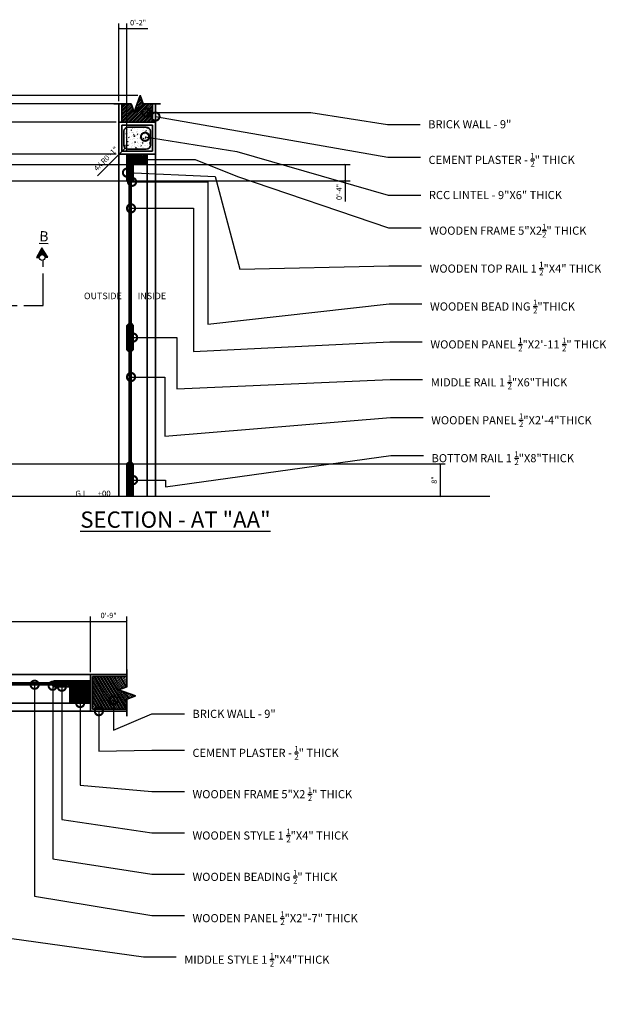
# Model space of a CAD drawing. Units: inches. Extents: x 1926 to 2169, y 1541 to 1783.
# Tile 3 of 3: x 2025 to 2169, y 1541 to 1783. Entities that reach past the tile are written whole.
import ezdxf
from ezdxf import colors
from ezdxf.entities.mleader import LeaderData, LeaderLine
from ezdxf.math import Vec2, Vec3

# ---------------------------------------------------------------- set-up
doc = ezdxf.new("R2010")
doc.units = ezdxf.units.IN
doc.linetypes.add('CENTER', pattern=[50.8, 31.75, -6.35, 6.35, -6.35])
for name, color, linetype, lineweight in [('A-ANNO-DIMS', 2, 'Continuous', 18), ('A-ANNO-SECT', 1, 'CENTER', 25), ('A-ANNO-SYMB', 1, 'Continuous', 25), ('A-ANNO-TEXT', 3, 'Continuous', 25), ('A-DETL', 7, 'Continuous', 35), ('A-DETL-PATT', 8, 'Continuous', 18)]:
    doc.layers.add(name, color=color, linetype=linetype, lineweight=lineweight)
doc.styles.get("Standard").update_dxf_attribs({"font": 'arial.ttf'})
doc.dimstyles.new('ISO-25', dxfattribs={"dimtxt": 1.3125, "dimasz": 0.375, "dimexe": 1.25, "dimexo": 0.625, "dimtad": 1, "dimzin": 3, "dimlunit": 4, "dimtxsty": 'Standard', "dimblk": 'ARCHTICK', "dimcen": 0.09, "dimadec": 0, "dimazin": 0, "dimtfac": 1, "dimtofl": 0, "dimtmove": 0, "dimatfit": 3, "dimfxl": 1, "dimarcsym": 0})

# ---------------------------------------------------------------- blocks, each defined once
blk = doc.blocks.new('_DotSmall')
at = {"color": 0, "linetype": 'ByBlock', "const_width": 0.5}
blk.add_lwpolyline([(-0.0625, 0, 1), (0.0625, 0, 1)], format="xyb", close=True, dxfattribs=at)
blk = doc.blocks.new('_ArchTick')
at = {"color": 0, "linetype": 'ByBlock', "const_width": 0.15}
blk.add_lwpolyline([(-0.5, -0.5), (0.5, 0.5)], dxfattribs=at)
blk = doc.blocks.new('*D24')
at = {"layer": 'A-ANNO-DIMS', "color": 0, "lineweight": -2, "transparency": 16777216}
for p, q in [((1974.41, 1673.81), (2129.74, 1673.81)), ((2128.49, 1673.81), (2128.49, 1665.81)), ((2134.77, 1665.81), (2127.24, 1665.81))]:
    blk.add_line(p, q, dxfattribs=at)
at = {"layer": 'DEFPOINTS', "color": 0, "transparency": 16777216}
for p in [(1973.78, 1673.81), (2128.49, 1665.81), (2135.4, 1665.81)]:
    blk.add_point(p, dxfattribs=at)
at = {"layer": 'A-ANNO-DIMS', "color": 0, "lineweight": -2, "transparency": 16777216, "xscale": 0.375, "yscale": 0.375, "zscale": 0.375}
for p, rotation in [((2128.49, 1673.81), 90), ((2128.49, 1665.81), 270)]:
    blk.add_blockref('_ArchTick', p, dxfattribs=dict(at, rotation=rotation))
at = {"layer": 'A-ANNO-DIMS', "color": 0, "transparency": 16777216, "insert": (2127.2, 1669.81), "char_height": 1.312, "attachment_point": 5, "rotation": 90}
blk.add_mtext('8"', dxfattribs=at)
blk = doc.blocks.new('*D28')
at = {"layer": 'A-ANNO-DIMS', "color": 0, "lineweight": -2, "transparency": 16777216}
for p, q in [((1966.66, 1749.81), (1954.13, 1749.81)), ((1955.38, 1749.81), (1955.38, 1665.81)), ((2140.71, 1665.81), (1954.13, 1665.81))]:
    blk.add_line(p, q, dxfattribs=at)
at = {"layer": 'DEFPOINTS', "color": 0, "transparency": 16777216}
for p in [(1967.28, 1749.81), (1955.38, 1665.81), (2141.33, 1665.81)]:
    blk.add_point(p, dxfattribs=at)
at = {"layer": 'A-ANNO-DIMS', "color": 0, "lineweight": -2, "transparency": 16777216, "xscale": 0.375, "yscale": 0.375, "zscale": 0.375}
for p, rotation in [((1955.38, 1749.81), 90), ((1955.38, 1665.81), 270)]:
    blk.add_blockref('_ArchTick', p, dxfattribs=dict(at, rotation=rotation))
at = {"layer": 'A-ANNO-DIMS', "color": 0, "transparency": 16777216, "insert": (1954.09, 1707.81), "char_height": 1.312, "attachment_point": 5, "rotation": 90}
blk.add_mtext('7\'-0"', dxfattribs=at)
blk = doc.blocks.new('*D32')
at = {"layer": 'A-ANNO-DIMS', "color": 0, "lineweight": -2, "transparency": 16777216}
for p, q in [((2013.41, 1747.31), (2106.38, 1747.31)), ((2105.13, 1747.31), (2105.13, 1743.31)), ((2009.41, 1743.31), (2106.38, 1743.31)), ((2105.13, 1743.31), (2105.13, 1738.19))]:
    blk.add_line(p, q, dxfattribs=at)
at = {"layer": 'DEFPOINTS', "color": 0, "transparency": 16777216}
for p in [(2012.78, 1747.31), (2008.78, 1743.31), (2105.13, 1743.31)]:
    blk.add_point(p, dxfattribs=at)
at = {"layer": 'A-ANNO-DIMS', "color": 0, "lineweight": -2, "transparency": 16777216, "xscale": 0.375, "yscale": 0.375, "zscale": 0.375}
for p, rotation in [((2105.13, 1747.31), 90), ((2105.13, 1743.31), 270)]:
    blk.add_blockref('_ArchTick', p, dxfattribs=dict(at, rotation=rotation))
at = {"layer": 'A-ANNO-DIMS', "color": 0, "transparency": 16777216, "insert": (2103.84, 1740.56), "char_height": 1.312, "attachment_point": 5, "rotation": 90}
blk.add_mtext('0\'-4"', dxfattribs=at)
blk = doc.blocks.new('*D35')
at = {"layer": 'A-ANNO-DIMS', "color": 0, "lineweight": -2, "transparency": 16777216}
for p, q in [((2054.17, 1764.25), (1935.51, 1764.25)), ((1936.76, 1665.81), (1936.76, 1764.25)), ((2048.92, 1665.81), (1935.51, 1665.81))]:
    blk.add_line(p, q, dxfattribs=at)
at = {"layer": 'DEFPOINTS', "color": 0, "transparency": 16777216}
for p in [(1936.76, 1764.25), (2054.79, 1764.25), (2049.54, 1665.81)]:
    blk.add_point(p, dxfattribs=at)
at = {"layer": 'A-ANNO-DIMS', "color": 0, "lineweight": -2, "transparency": 16777216, "xscale": 0.375, "yscale": 0.375, "zscale": 0.375}
for p, rotation in [((1936.76, 1764.25), 90), ((1936.76, 1665.81), 270)]:
    blk.add_blockref('_ArchTick', p, dxfattribs=dict(at, rotation=rotation))
at = {"layer": 'A-ANNO-DIMS', "color": 0, "transparency": 16777216, "insert": (1935.45, 1715.03), "char_height": 1.312, "attachment_point": 5, "rotation": 90}
blk.add_mtext('8\'-2 1/2"', dxfattribs=at)
blk = doc.blocks.new('*D36')
at = {"layer": 'A-ANNO-DIMS', "color": 0, "lineweight": -2, "transparency": 16777216}
for p, q in [((2049.54, 1762.82), (2049.54, 1781.93)), ((2049.54, 1780.68), (2051.54, 1780.68)), ((2051.54, 1750.43), (2051.54, 1781.93)), ((2051.54, 1780.68), (2056.65, 1780.68))]:
    blk.add_line(p, q, dxfattribs=at)
at = {"layer": 'DEFPOINTS', "color": 0, "transparency": 16777216}
for p in [(2051.54, 1780.68), (2049.54, 1762.19), (2051.54, 1749.81)]:
    blk.add_point(p, dxfattribs=at)
at = {"layer": 'A-ANNO-DIMS', "color": 0, "lineweight": -2, "transparency": 16777216, "xscale": 0.375, "yscale": 0.375, "zscale": 0.375, "rotation": 180}
blk.add_blockref('_ArchTick', (2049.54, 1780.68), dxfattribs=at)
at = {"layer": 'A-ANNO-DIMS', "color": 0, "lineweight": -2, "transparency": 16777216, "xscale": 0.375, "yscale": 0.375, "zscale": 0.375}
blk.add_blockref('_ArchTick', (2051.54, 1780.68), dxfattribs=at)
at = {"layer": 'A-ANNO-DIMS', "color": 0, "transparency": 16777216, "insert": (2054.28, 1781.97), "char_height": 1.312, "attachment_point": 5}
blk.add_mtext('0\'-2"', dxfattribs=at)
blk = doc.blocks.new('*D37')
at = {"layer": 'A-ANNO-DIMS', "color": 0, "lineweight": -2, "transparency": 16777216}
for p, q in [((2048.92, 1757.73), (1935.51, 1757.73)), ((1936.76, 1749.81), (1936.76, 1757.73)), ((2048.92, 1749.81), (1935.51, 1749.81))]:
    blk.add_line(p, q, dxfattribs=at)
at = {"layer": 'DEFPOINTS', "color": 0, "transparency": 16777216}
for p in [(1936.76, 1757.73), (2049.54, 1757.73), (2049.54, 1749.81)]:
    blk.add_point(p, dxfattribs=at)
at = {"layer": 'A-ANNO-DIMS', "color": 0, "lineweight": -2, "transparency": 16777216, "xscale": 0.375, "yscale": 0.375, "zscale": 0.375}
for p, rotation in [((1936.76, 1757.73), 90), ((1936.76, 1749.81), 270)]:
    blk.add_blockref('_ArchTick', p, dxfattribs=dict(at, rotation=rotation))
at = {"layer": 'A-ANNO-DIMS', "color": 0, "transparency": 16777216, "insert": (1935.46, 1753.77), "char_height": 1.312, "attachment_point": 5, "rotation": 90}
blk.add_mtext('0\'-8"', dxfattribs=at)
blk = doc.blocks.new('*D38')
at = {"layer": 'A-ANNO-DIMS', "color": 0, "lineweight": -2, "transparency": 16777216}
for p, q in [((1936.76, 1762.19), (1936.76, 1770.36)), ((2048.92, 1762.19), (1935.51, 1762.19)), ((1936.76, 1757.73), (1936.76, 1762.19)), ((2048.92, 1757.73), (1935.51, 1757.73))]:
    blk.add_line(p, q, dxfattribs=at)
at = {"layer": 'DEFPOINTS', "color": 0, "transparency": 16777216}
for p in [(1936.76, 1762.19), (2049.54, 1762.19), (2049.54, 1757.73)]:
    blk.add_point(p, dxfattribs=at)
at = {"layer": 'A-ANNO-DIMS', "color": 0, "lineweight": -2, "transparency": 16777216, "xscale": 0.375, "yscale": 0.375, "zscale": 0.375}
for p, rotation in [((1936.76, 1762.19), 90), ((1936.76, 1757.73), 270)]:
    blk.add_blockref('_ArchTick', p, dxfattribs=dict(at, rotation=rotation))
at = {"layer": 'A-ANNO-DIMS', "color": 0, "transparency": 16777216, "insert": (1935.45, 1766.46), "char_height": 1.312, "attachment_point": 5, "rotation": 90}
blk.add_mtext('0\'-4 1/2"', dxfattribs=at)
blk = doc.blocks.new('*D40')
at = {"layer": 'A-ANNO-DIMS', "color": 0, "lineweight": -2, "transparency": 16777216}
for p, q in [((1952.54, 1622.67), (1952.54, 1636.34)), ((1952.54, 1635.09), (2042.54, 1635.09)), ((2042.54, 1622.67), (2042.54, 1636.34))]:
    blk.add_line(p, q, dxfattribs=at)
at = {"layer": 'DEFPOINTS', "color": 0, "transparency": 16777216}
for p in [(2042.54, 1635.09), (1952.54, 1622.04), (2042.54, 1622.04)]:
    blk.add_point(p, dxfattribs=at)
at = {"layer": 'A-ANNO-DIMS', "color": 0, "lineweight": -2, "transparency": 16777216, "xscale": 0.375, "yscale": 0.375, "zscale": 0.375, "rotation": 180}
blk.add_blockref('_ArchTick', (1952.54, 1635.09), dxfattribs=at)
at = {"layer": 'A-ANNO-DIMS', "color": 0, "lineweight": -2, "transparency": 16777216, "xscale": 0.375, "yscale": 0.375, "zscale": 0.375}
blk.add_blockref('_ArchTick', (2042.54, 1635.09), dxfattribs=at)
at = {"layer": 'A-ANNO-DIMS', "color": 0, "transparency": 16777216, "insert": (1997.54, 1636.39), "char_height": 1.312, "attachment_point": 5}
blk.add_mtext('7\'-6"', dxfattribs=at)
blk = doc.blocks.new('*D41')
at = {"layer": 'A-ANNO-DIMS', "color": 0, "lineweight": -2, "transparency": 16777216}
for p, q in [((2042.54, 1622.67), (2042.54, 1636.34)), ((2042.54, 1635.09), (2051.54, 1635.09)), ((2051.54, 1622.67), (2051.54, 1636.34))]:
    blk.add_line(p, q, dxfattribs=at)
at = {"layer": 'DEFPOINTS', "color": 0, "transparency": 16777216}
for p in [(2051.54, 1635.09), (2042.54, 1622.04), (2051.54, 1622.04)]:
    blk.add_point(p, dxfattribs=at)
at = {"layer": 'A-ANNO-DIMS', "color": 0, "lineweight": -2, "transparency": 16777216, "xscale": 0.375, "yscale": 0.375, "zscale": 0.375, "rotation": 180}
blk.add_blockref('_ArchTick', (2042.54, 1635.09), dxfattribs=at)
at = {"layer": 'A-ANNO-DIMS', "color": 0, "lineweight": -2, "transparency": 16777216, "xscale": 0.375, "yscale": 0.375, "zscale": 0.375}
blk.add_blockref('_ArchTick', (2051.54, 1635.09), dxfattribs=at)
at = {"layer": 'A-ANNO-DIMS', "color": 0, "transparency": 16777216, "insert": (2047.04, 1636.39), "char_height": 1.312, "attachment_point": 5}
blk.add_mtext('0\'-9"', dxfattribs=at)
blk = doc.blocks.new('*D44')
at = {"layer": 'A-ANNO-DIMS', "color": 0, "lineweight": -2, "transparency": 16777216}
for p, q in [((2044.28, 1744.55), (2051.08, 1751.35)), ((2051.7, 1752.06), (2051.88, 1752.06)), ((2051.79, 1751.97), (2051.79, 1752.15))]:
    blk.add_line(p, q, dxfattribs=at)
at = {"layer": 'DEFPOINTS', "color": 0, "transparency": 16777216}
for p in [(2051.08, 1751.35), (2051.79, 1752.06)]:
    blk.add_point(p, dxfattribs=at)
at = {"layer": 'A-ANNO-DIMS', "color": 0, "lineweight": -2, "transparency": 16777216, "xscale": 0.375, "yscale": 0.375, "zscale": 0.375, "rotation": 45.01442306261743}
blk.add_blockref('_ArchTick', (2051.08, 1751.35), dxfattribs=at)
at = {"layer": 'A-ANNO-DIMS', "color": 0, "transparency": 16777216, "insert": (2046.5, 1748.6), "char_height": 1.312, "attachment_point": 5, "rotation": 45.0144}
blk.add_mtext('4X R0\'-1"', dxfattribs=at)

msp = doc.modelspace()

# ---------------------------------------------------------------- hatches: boundary and pattern name
at = {"layer": 'A-ANNO-SYMB'}
h = msp.add_hatch(color=256, dxfattribs=at)
h.dxf.hatch_style = 1
h.paths.add_polyline_path([(2031.409, 1724.514), (2032.103, 1724.566), (2030.609, 1726.871), (2029.289, 1724.461), (2029.985, 1724.461, -0.9636592)])
h = msp.add_hatch(dxfattribs=at)
h.set_pattern_fill('ANGLE', color=256, angle=90)
h.set_pattern_definition([(90, (3705.052, -295.39), (-6.985, 4e-16), [5.08, -1.905]), (180, (3705.052, -295.39), (-9e-16, -6.985), [5.08, -1.905])])
h.paths.add_polyline_path([(2054.821, 1719.063), (2053.501, 1716.653), (2054.197, 1716.653, -0.4142136), (2054.91, 1717.366, -0.3926966), (2055.621, 1716.706), (2056.315, 1716.757)])
at = {"layer": 'A-DETL-PATT'}
h = msp.add_hatch(dxfattribs=at)
h.set_pattern_fill('ANSI31', color=256, scale=0.1)
h.paths.add_polyline_path([(2053.29, 1760.129), (2052.54, 1762.19), (2050.29, 1762.19), (2050.29, 1757.726), (2057.79, 1757.726), (2057.79, 1762.19), (2055.54, 1762.19), (2054.79, 1764.251)])
h = msp.add_hatch(dxfattribs=at)
h.set_pattern_fill('AR-SAND', color=256)
h.paths.add_polyline_path([(2057.29, 1755.476, 0.4142136), (2056.29, 1756.476), (2051.79, 1756.476, 0.4142136), (2050.79, 1755.476), (2050.79, 1752.056, 0.4142136), (2051.79, 1751.056), (2056.29, 1751.056, 0.4142136), (2057.29, 1752.056)])
h = msp.add_hatch(dxfattribs=at)
h.set_pattern_fill('AR-CONC', color=256, scale=0.05)
h.paths.add_polyline_path([(2057.29, 1755.476, 0.4142136), (2056.29, 1756.476), (2051.79, 1756.476, 0.4142136), (2050.79, 1755.476), (2050.79, 1752.056, 0.4142136), (2051.79, 1751.056), (2056.29, 1751.056, 0.4142136), (2057.29, 1752.056)])
h = msp.add_hatch(dxfattribs=at)
h.set_pattern_fill('AR-CONC', color=256, scale=0.01)
h.paths.add_polyline_path([(2057.29, 1755.476, 0.4142136), (2056.29, 1756.476), (2051.79, 1756.476, 0.4142136), (2050.79, 1755.476), (2050.79, 1752.056, 0.4142136), (2051.79, 1751.056), (2056.29, 1751.056, 0.4142136), (2057.29, 1752.056)])
h = msp.add_hatch(dxfattribs=at)
h.set_pattern_fill('NET3', color=256, scale=0.1)
h.paths.add_polyline_path([(2051.54, 1701.806), (2052.04, 1701.306), (2052.04, 1674.306), (2051.54, 1673.806), (2051.54, 1665.806), (2053.04, 1665.806), (2053.04, 1673.806), (2052.54, 1674.306), (2052.54, 1701.306), (2053.04, 1701.806), (2053.04, 1707.806), (2052.54, 1708.306), (2052.54, 1742.806), (2053.04, 1743.306), (2053.04, 1747.306), (2051.54, 1747.306), (2051.54, 1743.306), (2052.04, 1742.806), (2052.04, 1708.306), (2051.54, 1707.806)])
h.paths.add_polyline_path([(2051.54, 1749.806), (2051.54, 1747.306), (2056.54, 1747.306), (2056.54, 1749.806)])
h = msp.add_hatch(dxfattribs=at)
h.set_pattern_fill('NET3', color=256, scale=0.1)
h.paths.add_polyline_path([(2001.54, 1620.543), (1997.54, 1620.543), (1997.54, 1619.043), (2001.54, 1619.043)])
h.paths.add_polyline_path([(2008.28, 1620.043), (2002.04, 1620.043), (2002.04, 1619.543), (2008.28, 1619.543)])
h.paths.add_polyline_path([(2002.04, 1620.043), (2001.54, 1620.543), (2001.54, 1619.043), (2002.04, 1619.543)])
h.paths.add_polyline_path([(2033.04, 1620.043), (2008.78, 1620.043), (2008.78, 1619.543), (2033.04, 1619.543)])
h.paths.add_polyline_path([(2037.54, 1620.543), (2033.54, 1620.543), (2033.54, 1619.043), (2037.54, 1619.043)])
h.paths.add_polyline_path([(2033.54, 1620.543), (2033.04, 1620.043), (2033.04, 1619.543), (2033.54, 1619.043)])
h.paths.add_polyline_path([(2042.54, 1620.543), (2037.54, 1620.543), (2037.54, 1615.043), (2042.54, 1615.043)])
h.paths.add_polyline_path([(2008.78, 1620.043), (2008.28, 1620.043), (2008.28, 1619.543), (2008.78, 1619.543)])
h = msp.add_hatch(dxfattribs=at)
h.set_pattern_fill('ANSI31', color=256, scale=0.1, angle=76)
h.paths.add_polyline_path([(2049.48, 1618.293), (2051.54, 1619.043), (2051.54, 1621.543), (2043.04, 1621.543), (2043.04, 1613.543), (2051.54, 1613.543), (2051.54, 1616.043), (2053.601, 1616.793)])

# ---------------------------------------------------------------- linework, layer by layer
at = {"layer": 'A-ANNO-SECT', "ltscale": 0.25}
msp.add_lwpolyline([(1949.966, 1720.956), (1949.966, 1712.639), (2030.915, 1712.639), (2030.915, 1723.782)], dxfattribs=at)
at = {"layer": 'A-ANNO-SYMB'}
msp.add_line((2093.331, 1665.806), (1950.218, 1665.806), dxfattribs=at)
msp.add_lwpolyline([(2031.409, 1724.514), (2032.103, 1724.566), (2030.609, 1726.871), (2029.289, 1724.461), (2029.985, 1724.461)], dxfattribs=at)
msp.add_circle((2030.698, 1724.461), 0.713, dxfattribs=at)
at = {"layer": 'A-DETL'}
for p, q in [((2049.54, 1762.19), (2049.54, 1665.806)), ((2050.29, 1762.19), (2050.29, 1757.726)), ((2050.29, 1762.19), (2050.29, 1757.726)), ((2057.79, 1762.19), (2057.79, 1757.726)), ((2057.79, 1762.19), (2057.79, 1757.726)), ((2058.54, 1762.19), (2058.54, 1665.806)), ((2049.54, 1757.726), (2058.54, 1757.726)), ((2050.29, 1756.976), (2057.79, 1756.976)), ((2050.29, 1756.976), (2050.29, 1750.556)), ((2057.79, 1756.976), (2057.79, 1750.556)), ((2058.54, 1749.806), (2049.54, 1749.806)), ((2057.79, 1750.556), (2050.29, 1750.556)), ((2051.54, 1743.306), (2051.54, 1747.306)), ((2053.04, 1743.306), (2053.04, 1747.306)), ((2056.54, 1747.306), (2056.54, 1665.806)), ((2052.04, 1742.806), (2051.54, 1743.306)), ((2052.04, 1742.806), (2052.04, 1708.306)), ((2052.04, 1708.306), (2052.04, 1742.806)), ((2052.54, 1742.806), (2053.04, 1743.306)), ((2052.54, 1742.806), (2052.54, 1708.306)), ((2052.54, 1708.306), (2052.54, 1742.806)), ((2052.04, 1708.306), (2051.54, 1707.806)), ((2051.54, 1707.806), (2051.54, 1701.806)), ((2052.54, 1708.306), (2053.04, 1707.806)), ((2053.04, 1707.806), (2053.04, 1701.806)), ((2052.04, 1701.306), (2051.54, 1701.806)), ((2052.04, 1701.306), (2052.04, 1674.306)), ((2053.04, 1701.806), (2052.54, 1701.306)), ((2052.54, 1701.306), (2052.54, 1674.306)), ((2052.04, 1674.306), (2051.54, 1673.806)), ((2051.54, 1673.806), (2051.54, 1665.806)), ((2052.54, 1674.306), (2053.04, 1673.806)), ((2053.04, 1673.806), (2053.04, 1665.806)), ((1991.28, 1622.043), (2051.54, 1622.043)), ((2033.04, 1620.043), (2033.54, 1620.543)), ((2037.54, 1620.543), (2033.54, 1620.543)), ((2033.54, 1619.043), (2033.54, 1620.543)), ((2037.54, 1615.043), (2037.54, 1620.543)), ((2037.54, 1620.543), (2042.54, 1620.543)), ((2042.54, 1613.043), (2042.54, 1622.043)), ((2043.04, 1613.543), (2043.04, 1621.543)), ((2043.04, 1621.543), (2051.54, 1621.543)), ((2033.04, 1620.043), (2002.04, 1620.043)), ((2033.04, 1619.543), (2002.04, 1619.543)), ((2033.04, 1619.543), (2033.04, 1620.043)), ((2033.54, 1619.043), (2033.04, 1619.543)), ((2037.54, 1619.043), (2033.54, 1619.043)), ((1957.54, 1615.043), (2037.54, 1615.043)), ((1991.28, 1613.043), (2051.54, 1613.043)), ((2037.54, 1615.043), (2042.54, 1615.043)), ((2043.04, 1613.543), (2051.54, 1613.543))]:
    msp.add_line(p, q, dxfattribs=at)
for points in [[(2059.79, 1762.19), (2055.54, 1762.19), (2054.79, 1764.251), (2053.29, 1760.129), (2052.54, 1762.19), (2048.29, 1762.19)], [(2051.79, 1756.476), (2056.29, 1756.476)], [(2050.79, 1752.056), (2050.79, 1755.476)], [(2057.29, 1755.476), (2057.29, 1752.056)], [(2056.29, 1751.056), (2051.79, 1751.056)], [(2051.54, 1611.793), (2051.54, 1616.043), (2053.601, 1616.793), (2049.48, 1618.293), (2051.54, 1619.043), (2051.54, 1623.293)]]:
    msp.add_lwpolyline(points, dxfattribs=at)
msp.add_lwpolyline([(2051.54, 1749.806), (2056.54, 1749.806), (2056.54, 1747.306), (2051.54, 1747.306)], close=True, dxfattribs=at)
for centre, start, end in [((2051.79, 1755.476), 90, 180), ((2056.29, 1755.476), 0, 90), ((2051.79, 1752.056), 180, 270), ((2056.29, 1752.056), 270, 0)]:
    msp.add_arc(centre, 1, start, end, dxfattribs=at)

# ---------------------------------------------------------------- texts
at = {"layer": 'A-ANNO-SYMB'}
msp.add_text('G.L      +00', height=1.40571, dxfattribs=at).set_placement((2038.869, 1665.806))
at = {"layer": 'A-ANNO-SYMB', "insert": (2030.066, 1730.978), "char_height": 2.5, "attachment_point": 1, "rotation": 357.55115}
msp.add_mtext_dynamic_manual_height_columns('{\\LB}', width=2.5, gutter_width=12.5, heights=[2.678], dxfattribs=at)
at = {"layer": 'A-ANNO-TEXT'}
for s, p in [('OUTSIDE', (2040.97, 1714.225)), ('INSIDE', (2054.173, 1714.225))]:
    msp.add_text(s, height=1.6109, dxfattribs=at).set_placement(p)
at = {"layer": 'A-ANNO-TEXT', "insert": (2040.071, 1662.1), "char_height": 4, "attachment_point": 1}
msp.add_mtext_dynamic_manual_height_columns('{\\LSECTION - AT "AA"}', width=57.58278, gutter_width=34.166, heights=[0], dxfattribs=at)

# ---------------------------------------------------------------- dimensions: what is measured, and where the dimension line sits
at = {"layer": 'A-ANNO-DIMS'}
for base, p1, p2, picture, middle in [((2051.54, 1780.678), (2049.54, 1762.19), (2051.54, 1749.806), '*D36', (2054.285, 1781.974)), ((2042.54, 1635.093), (1952.54, 1622.043), (2042.54, 1622.043), '*D40', (1997.54, 1636.388)), ((2051.54, 1635.093), (2042.54, 1622.043), (2051.54, 1622.043), '*D41', (2047.04, 1636.388))]:
    dim = msp.add_linear_dim(base=base, p1=p1, p2=p2, dimstyle='ISO-25', override={"dimdec": 1, "dimlfac": 1, "dimrnd": 0, "dimzin": 1, "dimdsep": 46, "dimlunit": 4, "dimfrac": 2}, dxfattribs=at)
    dim.commit()
    dim.dimension.update_dxf_attribs({"geometry": picture, "text_midpoint": middle})
for base, p1, p2, override, picture, middle in [((1936.757, 1762.19), (2049.54, 1757.726), (2049.54, 1762.19), {"dimdec": 1, "dimlfac": 1, "dimrnd": 0, "dimzin": 1, "dimdsep": 46, "dimlunit": 4, "dimfrac": 2}, '*D38', (1935.453, 1766.464)), ((1936.757, 1764.251), (2049.54, 1665.806), (2054.79, 1764.251), {"dimdec": 1, "dimlfac": 1, "dimrnd": 0, "dimzin": 1, "dimdsep": 46, "dimlunit": 4, "dimfrac": 2}, '*D35', (1935.453, 1715.028)), ((1936.757, 1757.726), (2049.54, 1749.806), (2049.54, 1757.726), {"dimdec": 1, "dimlfac": 1, "dimrnd": 0, "dimzin": 1, "dimdsep": 46, "dimlunit": 4, "dimfrac": 2}, '*D37', (1935.462, 1753.766)), ((1955.381, 1665.806), (1967.28, 1749.806), (2141.331, 1665.806), {"dimclrd": 0, "dimclre": 0, "dimclrt": 0}, '*D28', (1954.086, 1707.806)), ((2105.131, 1743.306), (2012.78, 1747.306), (2008.78, 1743.306), {"dimdec": 1, "dimlfac": 1, "dimrnd": 0, "dimzin": 1, "dimdsep": 46, "dimlunit": 4, "dimfrac": 2}, '*D32', (2103.836, 1740.561)), ((2128.49, 1665.806), (1973.78, 1673.806), (2135.399, 1665.806), {"dimclrd": 0, "dimclre": 0, "dimclrt": 0, "dimtmove": 1}, '*D24', (2127.195, 1669.806))]:
    dim = msp.add_linear_dim(base=base, p1=p1, p2=p2, angle=90, dimstyle='ISO-25', override=override, dxfattribs=at)
    dim.commit()
    dim.dimension.update_dxf_attribs({"geometry": picture, "text_midpoint": middle})
dim = msp.add_radius_dim(center=(2051.79, 1752.056), mpoint=(2051.083, 1751.348), text='4X <>', dimstyle='ISO-25', override={"dimdec": 1, "dimlfac": 1, "dimrnd": 0, "dimzin": 1, "dimdsep": 46, "dimlunit": 4, "dimfrac": 2}, dxfattribs=at)
dim.commit()
dim.dimension.update_dxf_attribs({"geometry": '*D44', "text_midpoint": (2046.503, 1748.597)})

# ---------------------------------------------------------------- leaders
at = {"layer": 'A-ANNO-TEXT'}
ml = msp.add_multileader_mtext('Standard', dxfattribs=at)
ml.set_content('BRICK WALL - 9"', color=256)
ml.set_leader_properties()
ml.set_arrow_properties(name='DOTSMALL')
ml.build(insert=Vec2(0, 0))
ctx = ml.context
ctx.base_point, ctx.char_height, ctx.plane_origin = Vec3(2123.551, 1757.17), 2, Vec3(2056.314, 1760.086)
notes = []
notes.append((ctx, [(0, (1, 1, 0), (2115.551, 1757.17), (1, 0), 8, [(0, [(2056.314, 1760.086), (2096.714, 1760.086), (2096.714, 1760.086)], 0, [])])]))
ctx.mtext.insert, ctx.mtext.flow_direction = Vec3(2125.551, 1758.187), 5
ml = msp.add_multileader_mtext('Standard', dxfattribs=at)
ml.set_content('\\A1;CEMENT PLASTER - {\\H0.7x;\\S1/2;}" THICK', color=256)
ml.set_leader_properties()
ml.set_arrow_properties(name='DOTSMALL')
ml.build(insert=Vec2(0, 0))
ctx = ml.context
ctx.base_point, ctx.char_height, ctx.plane_origin = Vec3(2123.633, 1749.102), 2, Vec3(2058.54, 1759.084)
notes.append((ctx, [(0, (1, 1, 0), (2115.633, 1749.102), (1, 0), 8, [(0, [(2058.54, 1759.084), (2087.098, 1754.137), (2087.098, 1754.137)], 0, [])])]))
ctx.mtext.insert, ctx.mtext.flow_direction = Vec3(2125.633, 1750.119), 5
ml = msp.add_multileader_mtext('Standard', dxfattribs=at)
ml.set_content('RCC LINTEL - 9"X6" THICK', color=256)
ml.set_leader_properties()
ml.set_arrow_properties(name='DOTSMALL')
ml.build(insert=Vec2(0, 0))
ctx = ml.context
ctx.base_point, ctx.char_height, ctx.plane_origin = Vec3(2123.728, 1739.79), 2, Vec3(2055.983, 1754.114)
notes.append((ctx, [(0, (1, 1, 0), (2115.728, 1739.79), (1, 0), 8, [(0, [(2055.983, 1754.114), (2078.525, 1750.524), (2078.525, 1750.524)], 0, [])])]))
ctx.mtext.insert, ctx.mtext.flow_direction = Vec3(2125.728, 1740.807), 5
ml = msp.add_multileader_mtext('Standard', dxfattribs=at)
ml.set_content('\\A1;WOODEN FRAME 5"X2{\\H0.7x;\\S1/2;}" THICK', color=256)
ml.set_leader_properties()
ml.set_arrow_properties(name='DOTSMALL')
ml.build(insert=Vec2(0, 0))
ctx = ml.context
ctx.base_point, ctx.char_height, ctx.plane_origin = Vec3(2123.81, 1731.722), 2, Vec3(2054.04, 1748.556)
notes.append((ctx, [(0, (1, 1, 0), (2115.81, 1731.722), (1, 0), 8, [(0, [(2054.04, 1748.556), (2068.303, 1748.556), (2078.682, 1744.399)], 0, [])])]))
ctx.mtext.insert, ctx.mtext.flow_direction = Vec3(2125.81, 1732.739), 5
ml = msp.add_multileader_mtext('Standard', dxfattribs=at)
ml.set_content('\\A1;WOODEN TOP RAIL 1 {\\H0.7x;\\S1/2;}"X4" THICK ', color=256)
ml.set_leader_properties()
ml.set_arrow_properties(name='DOTSMALL')
ml.build(insert=Vec2(0, 0))
ctx = ml.context
ctx.base_point, ctx.char_height, ctx.plane_origin = Vec3(2123.904, 1722.41), 2, Vec3(2051.54, 1745.306)
notes.append((ctx, [(0, (1, 1, 0), (2115.904, 1722.41), (1, 0), 8, [(0, [(2051.54, 1745.306), (2073.174, 1744.399), (2079.311, 1721.624)], 0, [])])]))
ctx.mtext.insert, ctx.mtext.flow_direction = Vec3(2125.904, 1723.427), 5
ml = msp.add_multileader_mtext('Standard', dxfattribs=at)
ml.set_content('\\A1;WOODEN BEAD ING {\\H0.7x;\\S1/2;}"THICK', color=256)
ml.set_leader_properties()
ml.set_arrow_properties(name='DOTSMALL')
ml.build(insert=Vec2(0, 0))
ctx = ml.context
ctx.base_point, ctx.char_height, ctx.plane_origin = Vec3(2123.999, 1713.097), 2, Vec3(2052.79, 1743.056)
notes.append((ctx, [(0, (1, 1, 0), (2115.999, 1713.097), (1, 0), 8, [(0, [(2052.79, 1743.056), (2071.445, 1743.056), (2071.445, 1708.117)], 0, [])])]))
ctx.mtext.insert, ctx.mtext.flow_direction = Vec3(2125.999, 1714.115), 5
ml = msp.add_multileader_mtext('Standard', dxfattribs=at)
ml.set_content('\\A1;WOODEN PANEL {\\H0.7x;\\S1/2;}"X2\'-11 {\\H0.7x;\\S1/2;}" THICK', color=256)
ml.set_leader_properties()
ml.set_arrow_properties(name='DOTSMALL')
ml.build(insert=Vec2(0, 0))
ctx = ml.context
ctx.base_point, ctx.char_height, ctx.plane_origin = Vec3(2124.094, 1703.785), 2, Vec3(2052.54, 1736.543)
notes.append((ctx, [(0, (1, 1, 0), (2116.094, 1703.785), (1, 0), 8, [(0, [(2052.54, 1736.543), (2067.866, 1736.543), (2067.866, 1701.363)], 0, [])])]))
ctx.mtext.insert, ctx.mtext.flow_direction = Vec3(2126.094, 1704.802), 5
ml = msp.add_multileader_mtext('Standard', dxfattribs=at)
ml.set_content('\\A1;MIDDLE RAIL 1 {\\H0.7x;\\S1/2;}"X6"THICK', color=256)
ml.set_leader_properties()
ml.set_arrow_properties(name='DOTSMALL')
ml.build(insert=Vec2(0, 0))
ctx = ml.context
ctx.base_point, ctx.char_height, ctx.plane_origin = Vec3(2124.188, 1694.473), 2, Vec3(2053.04, 1704.806)
notes.append((ctx, [(0, (1, 1, 0), (2116.188, 1694.473), (1, 0), 8, [(0, [(2053.04, 1704.806), (2063.792, 1704.806), (2063.792, 1692.253)], 0, [])])]))
ctx.mtext.insert, ctx.mtext.flow_direction = Vec3(2126.188, 1695.49), 5
ml = msp.add_multileader_mtext('Standard', dxfattribs=at)
ml.set_content('\\A1;WOODEN PANEL {\\H0.7x;\\S1/2;}"X2\'-4"THICK', color=256)
ml.set_leader_properties()
ml.set_arrow_properties(name='DOTSMALL')
ml.build(insert=Vec2(0, 0))
ctx = ml.context
ctx.base_point, ctx.char_height, ctx.plane_origin = Vec3(2124.283, 1685.161), 2, Vec3(2052.54, 1695.113)
notes.append((ctx, [(0, (1, 1, 0), (2116.283, 1685.161), (1, 0), 8, [(0, [(2052.54, 1695.113), (2060.847, 1695.113), (2060.847, 1680.63)], 0, [])])]))
ctx.mtext.insert, ctx.mtext.flow_direction = Vec3(2126.283, 1686.178), 5
ml = msp.add_multileader_mtext('Standard', dxfattribs=at)
ml.set_content('\\A1;BOTTOM RAIL 1 {\\H0.7x;\\S1/2;}"X8"THICK', color=256)
ml.set_leader_properties()
ml.set_arrow_properties(name='DOTSMALL')
ml.build(insert=Vec2(0, 0))
ctx = ml.context
ctx.base_point, ctx.char_height, ctx.plane_origin = Vec3(2124.378, 1675.849), 2, Vec3(2053.04, 1669.806)
notes.append((ctx, [(0, (1, 1, 0), (2116.378, 1675.849), (1, 0), 8, [(0, [(2053.04, 1669.806), (2061.002, 1669.806), (2061.002, 1668.169)], 0, [])])]))
ctx.mtext.insert, ctx.mtext.flow_direction = Vec3(2126.378, 1676.866), 5
ml = msp.add_multileader_mtext('Standard', dxfattribs=at)
ml.set_content('\\A1;MIDDLE STYLE 1 {\\H0.7x;\\S1/2;}"X4"THICK', color=256)
ml.set_leader_properties()
ml.set_arrow_properties(name='DOTSMALL')
ml.build(insert=Vec2(0, 0))
ctx = ml.context
ctx.base_point, ctx.char_height, ctx.plane_origin = Vec3(2063.638, 1552.694), 2, Vec3(1999.54, 1619.043)
notes.append((ctx, [(0, (1, 1, 0), (2055.638, 1552.694), (1, 0), 8, [(0, [(1999.54, 1619.043), (2004.296, 1609.195), (2009.741, 1559.148)], 0, [])])]))
ctx.mtext.insert, ctx.mtext.flow_direction = Vec3(2065.638, 1553.711), 5
ml = msp.add_multileader_mtext('Standard', dxfattribs=at)
ml.set_content('\\A1;WOODEN PANEL {\\H0.7x;\\S1/2;}"X2"-7" THICK', color=256)
ml.set_leader_properties()
ml.set_arrow_properties(name='DOTSMALL')
ml.build(insert=Vec2(0, 0))
ctx = ml.context
ctx.base_point, ctx.char_height, ctx.plane_origin = Vec3(2065.638, 1562.881), 2, Vec3(2028.859, 1619.543)
notes.append((ctx, [(0, (1, 1, 0), (2057.638, 1562.881), (1, 0), 8, [(0, [(2028.859, 1619.543), (2028.859, 1567.64)], 0, [])])]))
ctx.mtext.insert, ctx.mtext.flow_direction = Vec3(2067.638, 1563.898), 5
ml = msp.add_multileader_mtext('Standard', dxfattribs=at)
ml.set_content('\\A1;WOODEN BEADING {\\H0.7x;\\S1/2;}" THICK', color=256)
ml.set_leader_properties()
ml.set_arrow_properties(name='DOTSMALL')
ml.build(insert=Vec2(0, 0))
ctx = ml.context
ctx.base_point, ctx.char_height, ctx.plane_origin = Vec3(2065.638, 1573.03), 2, Vec3(2033.29, 1619.293)
notes.append((ctx, [(0, (1, 1, 0), (2057.638, 1573.03), (1, 0), 8, [(0, [(2033.29, 1619.293), (2033.29, 1576.773)], 0, [])])]))
ctx.mtext.insert, ctx.mtext.flow_direction = Vec3(2067.638, 1574.047), 5
ml = msp.add_multileader_mtext('Standard', dxfattribs=at)
ml.set_content('\\A1;WOODEN STYLE 1 {\\H0.7x;\\S1/2;}"X4" THICK', color=256)
ml.set_leader_properties()
ml.set_arrow_properties(name='DOTSMALL')
ml.build(insert=Vec2(0, 0))
ctx = ml.context
ctx.base_point, ctx.char_height, ctx.plane_origin = Vec3(2065.638, 1583.179), 2, Vec3(2035.54, 1619.043)
notes.append((ctx, [(0, (1, 1, 0), (2057.638, 1583.179), (1, 0), 8, [(0, [(2035.54, 1619.043), (2035.54, 1586.452)], 0, [])])]))
ctx.mtext.insert, ctx.mtext.flow_direction = Vec3(2067.638, 1584.196), 5
ml = msp.add_multileader_mtext('Standard', dxfattribs=at)
ml.set_content('\\A1;WOODEN FRAME 5"X2 {\\H0.7x;\\S1/2;}" THICK', color=256)
ml.set_leader_properties()
ml.set_arrow_properties(name='DOTSMALL')
ml.build(insert=Vec2(0, 0))
ctx = ml.context
ctx.base_point, ctx.char_height, ctx.plane_origin = Vec3(2065.638, 1593.328), 2, Vec3(2040.04, 1615.043)
notes.append((ctx, [(0, (1, 1, 0), (2057.638, 1593.328), (1, 0), 8, [(0, [(2040.04, 1615.043), (2040.04, 1594.902)], 0, [])])]))
ctx.mtext.insert, ctx.mtext.flow_direction = Vec3(2067.638, 1594.345), 5
ml = msp.add_multileader_mtext('Standard', dxfattribs=at)
ml.set_content('BRICK WALL - 9"', color=256)
ml.set_leader_properties()
ml.set_arrow_properties(name='DOTSMALL')
ml.build(insert=Vec2(0, 0))
ctx = ml.context
ctx.base_point, ctx.char_height, ctx.plane_origin = Vec3(2065.638, 1612.381), 2, Vec3(2048.243, 1615.718)
notes.append((ctx, [(0, (1, 1, 0), (2057.638, 1612.381), (1, 0), 8, [(0, [(2048.243, 1615.718), (2048.243, 1608.385)], 0, [])])]))
ctx.mtext.insert, ctx.mtext.flow_direction = Vec3(2067.638, 1613.398), 5
ml = msp.add_multileader_mtext('Standard', dxfattribs=at)
ml.set_content('\\A1;CEMENT PLASTER - {\\H0.7x;\\S1/2;}" THICK', color=256)
ml.set_leader_properties()
ml.set_arrow_properties(name='DOTSMALL')
ml.build(insert=Vec2(0, 0))
ctx = ml.context
ctx.base_point, ctx.char_height, ctx.plane_origin = Vec3(2065.638, 1603.477), 2, Vec3(2044.641, 1613.043)
notes.append((ctx, [(0, (1, 1, 0), (2057.638, 1603.477), (1, 0), 8, [(0, [(2044.641, 1613.043), (2044.641, 1603.264)], 0, [])])]))
ctx.mtext.insert, ctx.mtext.flow_direction = Vec3(2067.638, 1604.494), 5
for ctx, leaders in notes:
    for number, flags, end, landing, length, lines in leaders:
        leader = LeaderData()
        leader.index, (leader.has_last_leader_line, leader.has_dogleg_vector, leader.attachment_direction) = number, flags
        leader.last_leader_point, leader.dogleg_vector, leader.dogleg_length = Vec3(end), Vec3(landing), length
        for number, points, colour, breaks in lines:
            line = LeaderLine()
            line.index, line.vertices, line.color, line.breaks = number, Vec3.list(points), colors.encode_raw_color(colour), breaks
            leader.lines.append(line)
        ctx.leaders.append(leader)

doc.saveas('drawing.dxf')
